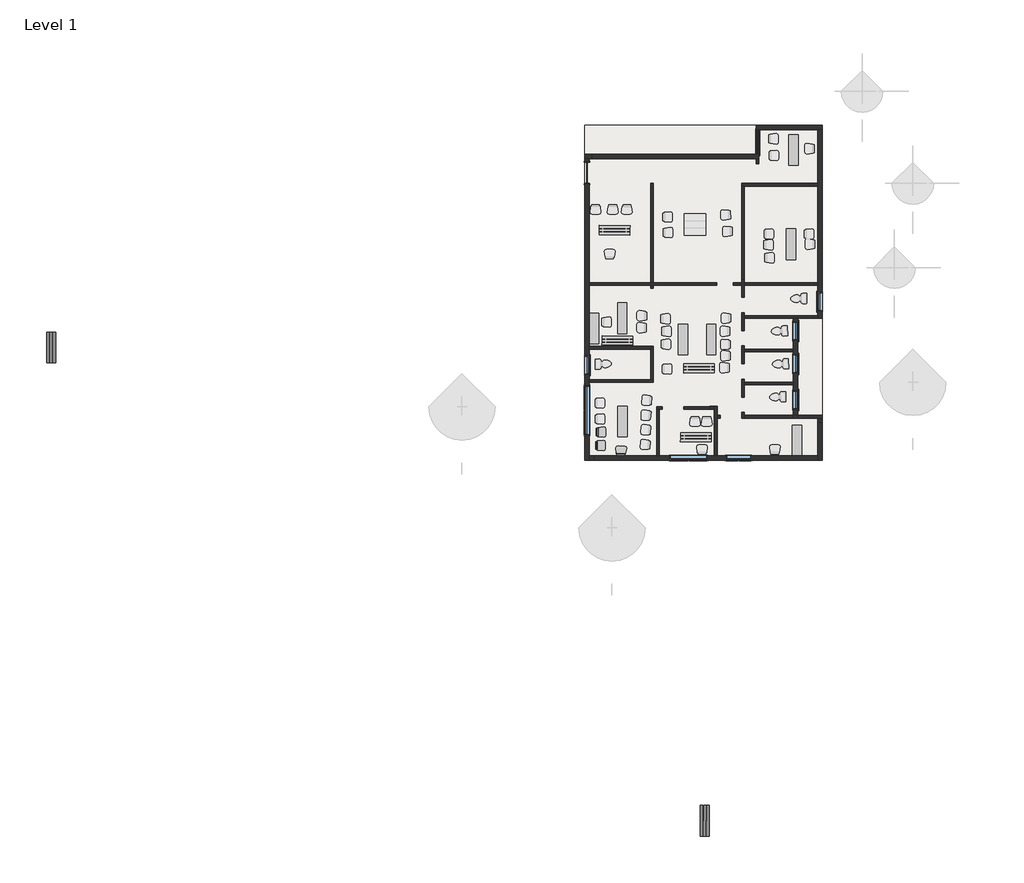
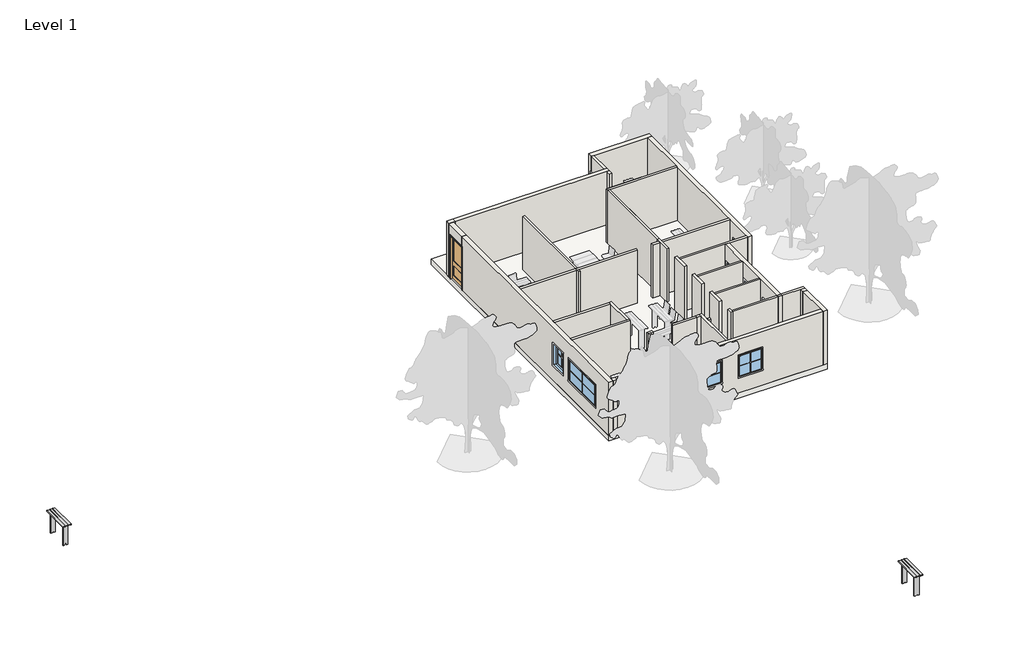
# One storey, part 1 of 2: 46 walls, 9 windows, 5 furniture elements, 1 door, 1 slab.
"""IFC4 building model written with IfcOpenShell, lengths in millimetres."""

from ifc_helpers import new_model, si_unit, frame, origin, origin_with_axes, place, context, project, spatial, polyline, outline, extrude, faceted_brep, transform, mapped, element, save
from components import door_07f5c701, furniture_f7008d8d, chair_desk_chair_desk_7ad88740, window_fixed_2_d4a0c5b4, window_fixed_3_f41792bd, window_fixed_5_cc3256ea, window_fixed_8_9704bb16, window_fixed_9_035f8342

model = new_model("IFC4")

# Units and contexts
model_context = context("Model", 3, world=origin())
ifc_project = project(units=[si_unit("LENGTHUNIT", "METRE", prefix="MILLI")], contexts=[model_context])

# Site, building, storey
site = spatial("IfcSite", under=ifc_project)
building = spatial("IfcBuilding", under=site)
storey = spatial("IfcBuildingStorey", under=building, Name="Level 1", Elevation=0.0)

# Door
placement = place(None, origin())
door_shape = door_07f5c701(model_context)
element("IfcDoor", 1, ObjectType="Door-Interior-Single-Pocket-2_Panel-Wood : 42\" x 96\"", at=placement, inside=storey, context=model_context, shape_type="MappedRepresentation", body=[
    mapped(door_shape, transform((1384.3, 26568.4, 0.0), x_axis=(0.0, -1.0, 0.0), y_axis=(1.0, 0.0, 0.0), z_axis=(0.0, 0.0, 1.0))),
])

# Furniture
furniture_shape = furniture_f7008d8d(model_context)
element("IfcFurniture", 2, ObjectType="Bench-Locker Room : 48\" x 18\" x 14\"", at=placement, inside=storey, context=model_context, shape_type="MappedRepresentation", body=[
    mapped(furniture_shape, transform((-25423.3983688, 18061.4041391, 0.0), x_axis=(0.0, 1.0, 0.0), y_axis=(-1.0, 0.0, 0.0), z_axis=(0.0, 0.0, 1.0))),
])
element("IfcFurniture", 3, ObjectType="Bench-Locker Room : 48\" x 18\" x 14\"", at=placement, inside=storey, context=model_context, shape_type="MappedRepresentation", body=[
    mapped(furniture_shape, transform((7417.2524983, -5769.7183685, 0.0), x_axis=(-0.004811439454211425, -0.9999884249581985, 0.0), y_axis=(0.9999884249581985, -0.004811439454211425, 0.0), z_axis=(0.0, 0.0, 1.0))),
])
chair_desk_chair_desk_shape = chair_desk_chair_desk_7ad88740(model_context)
element("IfcFurniture", 4, ObjectType="Chair-Desk : Chair-Desk", at=placement, inside=storey, context=model_context, shape_type="MappedRepresentation", body=[
    mapped(chair_desk_chair_desk_shape, transform((1917.2646776, 13701.8247599, 0.0), x_axis=(0.0, -1.0, 0.0), y_axis=(1.0, 0.0, 0.0), z_axis=(0.0, 0.0, 1.0))),
])
element("IfcFurniture", 5, ObjectType="Chair-Desk : Chair-Desk", at=placement, inside=storey, context=model_context, shape_type="MappedRepresentation", body=[
    mapped(chair_desk_chair_desk_shape, transform((1889.1210098, 13035.1530931, 0.0), x_axis=(0.0, -1.0, 0.0), y_axis=(1.0, 0.0, 0.0), z_axis=(0.0, 0.0, 1.0))),
])
element("IfcFurniture", 6, ObjectType="Chair-Desk : Chair-Desk", at=placement, inside=storey, context=model_context, shape_type="MappedRepresentation", body=[
    mapped(chair_desk_chair_desk_shape, transform((3069.589979, 12617.2374558, 0.0), x_axis=(0.9977976465817522, -0.066331413944804, 0.0), y_axis=(0.066331413944804, 0.9977976465817522, 0.0), z_axis=(0.0, 0.0, 1.0))),
])

# Slab
element("IfcSlab", 7, ObjectType="Generic - 12\"", at=placement, inside=storey, context=model_context, shape_type="SweptSolid", body=[
    extrude(outline(polyline([(1270.0, 28956.0), (13081.0, 28956.0), (13081.0, 12293.6), (1270.0, 12293.6), (1270.0, 28956.0)])), frame((0.0, 0.0, -304.8), z_axis=(0.0, 0.0, 1.0), x_axis=(1.0, 0.0, 0.0)), (0.0, 0.0, 1.0), 304.8),
])

# Walls
element("IfcWall", 8, at=placement, inside=storey, context=model_context, shape_type="Brep", body=[
    faceted_brep([(7493.0, 14985.1789567, 0.0), (7493.0, 14960.6, 0.0), (7493.0, 14833.6, 0.0), (7493.0, 14833.6, 3048.0), (7493.0, 14960.6, 3048.0), (7493.0, 14985.1789567, 3048.0), (7721.6, 14985.1789567, 0.0), (7721.6, 14985.1789567, 3048.0), (7721.6, 14833.6, 3048.0), (7721.6, 14833.6, 0.0)], [[[0, 1, 2, 3, 4, 5]], [[6, 7, 8, 9]], [[2, 1, 0, 6, 9]], [[0, 5, 7, 6]], [[3, 2, 9, 8]], [[5, 4, 3, 8, 7]]]),
])
element("IfcWall", 9, at=placement, inside=storey, context=model_context, shape_type="SweptSolid", body=[
    extrude(outline(polyline([(7493.0, 14960.6), (7493.0, 14985.1789567), (7721.6, 14985.1789567), (7721.6, 14960.6), (7493.0, 14960.6)])), origin_with_axes(), (0.0, 0.0, 1.0), 3048.0),
])
element("IfcWall", 10, ObjectType="5\"", at=placement, inside=storey, context=model_context, shape_type="Brep", body=[
    faceted_brep([(12852.4, 19481.8, 0.0), (9194.8, 19481.8, 0.0), (9194.8, 19481.8, 3048.0), (12852.4, 19481.8, 3048.0), (12852.4, 19354.8, 0.0), (12852.4, 19354.8, 3048.0), (11861.8, 19354.8, 3048.0), (11633.2, 19354.8, 3048.0), (9194.8, 19354.8, 3048.0), (9194.8, 19354.8, 0.0), (11633.2, 19354.8, 0.0), (11861.8, 19354.8, 0.0)], [[[0, 1, 2, 3]], [[4, 5, 6, 7, 8, 9, 10, 11]], [[1, 0, 4, 11, 10, 9]], [[0, 3, 5, 4]], [[2, 1, 9, 8]], [[3, 2, 8, 7, 6, 5]]]),
])
element("IfcWall", 11, ObjectType="5\"", at=placement, inside=storey, context=model_context, shape_type="Brep", body=[
    faceted_brep([(9067.8, 19634.2, 0.0), (9067.8, 18745.2, 0.0), (9067.8, 18745.2, 3048.0), (9067.8, 19634.2, 3048.0), (9194.8, 19634.2, 0.0), (9194.8, 19634.2, 3048.0), (9194.8, 19481.8, 3048.0), (9194.8, 19354.8, 3048.0), (9194.8, 18745.2, 3048.0), (9194.8, 18745.2, 0.0), (9194.8, 19354.8, 0.0), (9194.8, 19481.8, 0.0)], [[[0, 1, 2, 3]], [[4, 5, 6, 7, 8, 9, 10, 11]], [[1, 0, 4, 11, 10, 9]], [[2, 1, 9, 8]], [[0, 3, 5, 4]], [[3, 2, 8, 7, 6, 5]]]),
])
element("IfcWall", 12, ObjectType="5\"", at=placement, inside=storey, context=model_context, shape_type="SweptSolid", body=[
    extrude(outline(polyline([(9067.8, 20396.2), (9067.8, 21285.2), (9194.8, 21285.2), (9194.8, 20396.2), (9067.8, 20396.2)])), origin_with_axes(), (0.0, 0.0, 1.0), 3048.0),
])
element("IfcWall", 13, ObjectType="5\"", at=placement, inside=storey, context=model_context, shape_type="Brep", body=[
    faceted_brep([(12852.4, 26060.4, 0.0), (9067.8, 26060.4, 0.0), (9067.8, 26060.4, 3048.0), (12852.4, 26060.4, 3048.0), (12852.4, 25933.4, 0.0), (12852.4, 25933.4, 3048.0), (9194.8, 25933.4, 3048.0), (9067.8, 25933.4, 3048.0), (9067.8, 25933.4, 0.0), (9194.8, 25933.4, 0.0)], [[[0, 1, 2, 3]], [[4, 5, 6, 7, 8, 9]], [[1, 0, 4, 9, 8]], [[0, 3, 5, 4]], [[2, 1, 8, 7]], [[3, 2, 7, 6, 5]]]),
])
element("IfcWall", 14, ObjectType="5\"", at=placement, inside=storey, context=model_context, shape_type="SweptSolid", body=[
    extrude(outline(polyline([(9067.8, 22352.0), (9067.8, 25933.4), (9194.8, 25933.4), (9194.8, 22352.0), (9067.8, 22352.0)])), origin_with_axes(), (0.0, 0.0, 1.0), 3048.0),
])
element("IfcWall", 15, ObjectType="5\"", at=placement, inside=storey, context=model_context, shape_type="SweptSolid", body=[
    extrude(outline(polyline([(9194.8, 17830.8), (11633.2, 17830.8), (11633.2, 17703.8), (9194.8, 17703.8), (9194.8, 17830.8)])), origin_with_axes(), (0.0, 0.0, 1.0), 3048.0),
])
element("IfcWall", 16, ObjectType="5\"", at=placement, inside=storey, context=model_context, shape_type="Brep", body=[
    faceted_brep([(9067.8, 17983.2, 0.0), (9067.8, 17094.2, 0.0), (9067.8, 17094.2, 3048.0), (9067.8, 17983.2, 3048.0), (9194.8, 17983.2, 0.0), (9194.8, 17983.2, 3048.0), (9194.8, 17830.8, 3048.0), (9194.8, 17703.8, 3048.0), (9194.8, 17094.2, 3048.0), (9194.8, 17094.2, 0.0), (9194.8, 17703.8, 0.0), (9194.8, 17830.8, 0.0)], [[[0, 1, 2, 3]], [[4, 5, 6, 7, 8, 9, 10, 11]], [[1, 0, 4, 11, 10, 9]], [[2, 1, 9, 8]], [[0, 3, 5, 4]], [[3, 2, 8, 7, 6, 5]]]),
])
element("IfcWall", 17, ObjectType="5\"", at=placement, inside=storey, context=model_context, shape_type="SweptSolid", body=[
    extrude(outline(polyline([(9194.8, 16179.8), (11633.2, 16179.8), (11633.2, 16052.8), (9194.8, 16052.8), (9194.8, 16179.8)])), origin_with_axes(), (0.0, 0.0, 1.0), 3048.0),
])
element("IfcWall", 18, ObjectType="5\"", at=placement, inside=storey, context=model_context, shape_type="Brep", body=[
    faceted_brep([(9067.8, 16332.2, 0.0), (9067.8, 15443.2, 0.0), (9067.8, 15443.2, 3048.0), (9067.8, 16332.2, 3048.0), (9194.8, 16332.2, 0.0), (9194.8, 16332.2, 3048.0), (9194.8, 16179.8, 3048.0), (9194.8, 16052.8, 3048.0), (9194.8, 15443.2, 3048.0), (9194.8, 15443.2, 0.0), (9194.8, 16052.8, 0.0), (9194.8, 16179.8, 0.0)], [[[0, 1, 2, 3]], [[4, 5, 6, 7, 8, 9, 10, 11]], [[1, 0, 4, 11, 10, 9]], [[2, 1, 9, 8]], [[0, 3, 5, 4]], [[3, 2, 8, 7, 6, 5]]]),
])
element("IfcWall", 19, ObjectType="5\"", at=placement, inside=storey, context=model_context, shape_type="Brep", body=[
    faceted_brep([(13081.0, 14528.8, 0.0), (11861.8, 14528.8, 0.0), (11633.2, 14528.8, 0.0), (9194.8, 14528.8, 0.0), (9194.8, 14528.8, 3048.0), (11633.2, 14528.8, 3048.0), (11861.8, 14528.8, 3048.0), (13081.0, 14528.8, 3048.0), (13081.0, 14401.8, 0.0), (13081.0, 14401.8, 3048.0), (9194.8, 14401.8, 3048.0), (9194.8, 14401.8, 0.0)], [[[0, 1, 2, 3, 4, 5, 6, 7]], [[8, 9, 10, 11]], [[3, 2, 1, 0, 8, 11]], [[0, 7, 9, 8]], [[4, 3, 11, 10]], [[7, 6, 5, 4, 10, 9]]]),
])
element("IfcWall", 20, ObjectType="5\"", at=placement, inside=storey, context=model_context, shape_type="Brep", body=[
    faceted_brep([(9067.8, 14681.2, 0.0), (9067.8, 14401.8, 0.0), (9067.8, 14401.8, 3048.0), (9067.8, 14681.2, 3048.0), (9194.8, 14681.2, 0.0), (9194.8, 14681.2, 3048.0), (9194.8, 14528.8, 3048.0), (9194.8, 14401.8, 3048.0), (9194.8, 14401.8, 0.0), (9194.8, 14528.8, 0.0)], [[[0, 1, 2, 3]], [[4, 5, 6, 7, 8, 9]], [[1, 0, 4, 9, 8]], [[0, 3, 5, 4]], [[2, 1, 8, 7]], [[3, 2, 7, 6, 5]]]),
])
element("IfcWall", 21, ObjectType="5\"", at=placement, inside=storey, context=model_context, shape_type="SweptSolid", body=[
    extrude(outline(polyline([(1498.6, 21132.8), (7844.2592865, 21132.8), (7844.2592865, 21005.8), (1498.6, 21005.8), (1498.6, 21132.8)])), origin_with_axes(), (0.0, 0.0, 1.0), 3048.0),
])
element("IfcWall", 22, ObjectType="5\"", at=placement, inside=storey, context=model_context, shape_type="SweptSolid", body=[
    extrude(outline(polyline([(4546.6, 20853.4004015), (4546.6, 26060.4), (4673.6, 26060.4), (4673.6, 20853.4004015), (4546.6, 20853.4004015)])), origin_with_axes(), (0.0, 0.0, 1.0), 3048.0),
])
element("IfcWall", 23, ObjectType="5\"", at=placement, inside=storey, context=model_context, shape_type="Brep", body=[
    faceted_brep([(5130.8, 14960.6, 0.0), (4851.4, 14960.6, 0.0), (4851.4, 14960.6, 3048.0), (5130.8, 14960.6, 3048.0), (5130.8, 14833.6, 0.0), (5130.8, 14833.6, 3048.0), (4978.4, 14833.6, 3048.0), (4851.4, 14833.6, 3048.0), (4851.4, 14833.6, 0.0), (4978.4, 14833.6, 0.0)], [[[0, 1, 2, 3]], [[4, 5, 6, 7, 8, 9]], [[1, 0, 4, 9, 8]], [[0, 3, 5, 4]], [[2, 1, 8, 7]], [[3, 2, 7, 6, 5]]]),
])
element("IfcWall", 24, ObjectType="5\"", at=placement, inside=storey, context=model_context, shape_type="SweptSolid", body=[
    extrude(outline(polyline([(4851.4, 12522.2), (4851.4, 14833.6), (4978.4, 14833.6), (4978.4, 12522.2), (4851.4, 12522.2)])), origin_with_axes(), (0.0, 0.0, 1.0), 3048.0),
])
element("IfcWall", 25, ObjectType="5\"", at=placement, inside=storey, context=model_context, shape_type="Brep", body=[
    faceted_brep([(7848.6, 12522.2, 0.0), (7848.6, 14401.8, 0.0), (7848.6, 14528.8, 0.0), (7848.6, 14985.1789567, 0.0), (7848.6, 14985.1789567, 3048.0), (7848.6, 14528.8, 3048.0), (7848.6, 14401.8, 3048.0), (7848.6, 12522.2, 3048.0), (7721.6, 12522.2, 0.0), (7721.6, 12522.2, 3048.0), (7721.6, 14985.1789567, 3048.0), (7721.6, 14985.1789567, 0.0)], [[[0, 1, 2, 3, 4, 5, 6, 7]], [[8, 9, 10, 11]], [[3, 2, 1, 0, 8, 11]], [[4, 3, 11, 10]], [[0, 7, 9, 8]], [[7, 6, 5, 4, 10, 9]]]),
])
element("IfcWall", 26, ObjectType="5\"", at=placement, inside=storey, context=model_context, shape_type="SweptSolid", body=[
    extrude(outline(polyline([(6197.6, 14960.6), (7493.0, 14960.6), (7493.0, 14833.6), (6197.6, 14833.6), (6197.6, 14960.6)])), origin_with_axes(), (0.0, 0.0, 1.0), 3048.0),
])
element("IfcWall", 27, ObjectType="5\"", at=placement, inside=storey, context=model_context, shape_type="SweptSolid", body=[
    extrude(outline(polyline([(9804.4, 27508.2), (9804.4, 28727.4), (9931.4, 28727.4), (9931.4, 27508.2), (9804.4, 27508.2)])), origin_with_axes(), (0.0, 0.0, 1.0), 914.4),
    extrude(outline(polyline([(9804.4, 27508.2), (9804.4, 28727.4), (9931.4, 28727.4), (9931.4, 27508.2), (9804.4, 27508.2)])), frame((0.0, 0.0, 2133.6), z_axis=(0.0, 0.0, 1.0), x_axis=(1.0, 0.0, 0.0)), (0.0, 0.0, 1.0), 914.4),
])
element("IfcWall", 28, ObjectType="5\"", at=placement, inside=storey, context=model_context, shape_type="SweptSolid", body=[
    extrude(outline(polyline([(7874.0, 14401.8), (7874.0, 14528.8), (8001.0, 14528.8), (8001.0, 14401.8), (7874.0, 14401.8)])), origin_with_axes(), (0.0, 0.0, 1.0), 3048.0),
])
element("IfcWall", 29, ObjectType="5\"", at=placement, inside=storey, context=model_context, shape_type="SweptSolid", body=[
    extrude(outline(polyline([(7848.6, 14528.8), (7874.0, 14528.8), (7874.0, 14401.8), (7848.6, 14401.8), (7848.6, 14528.8)])), origin_with_axes(), (0.0, 0.0, 1.0), 3048.0),
])
element("IfcWall", 30, ObjectType="9\"", at=placement, inside=storey, context=model_context, shape_type="SweptSolid", body=[
    extrude(outline(polyline([(27279.6, 3048.0), (27279.6, 0.0), (27127.2, 0.0), (27127.2, 2463.8), (26060.4, 2463.8), (26060.4, 3048.0), (27279.6, 3048.0)])), frame((1270.0, 0.0, 0.0), z_axis=(1.0, 0.0, 0.0), x_axis=(0.0, 1.0, 0.0)), (0.0, 0.0, 1.0), 228.6),
])
element("IfcWall", 31, ObjectType="9\"", at=placement, inside=storey, context=model_context, shape_type="Brep", body=[
    faceted_brep([(1270.0, 12293.6, 0.0), (1270.0, 12293.6, 3048.0), (1270.0, 26060.4, 3048.0), (1270.0, 26060.4, 2463.8), (1270.0, 26035.0, 2463.8), (1270.0, 26035.0, 0.0), (1270.0, 16572.1631818, 2133.6), (1270.0, 16572.1631818, 914.4), (1270.0, 17486.5631818, 914.4), (1270.0, 17486.5631818, 2133.6), (1270.0, 16002.6980131, 2133.6), (1270.0, 13564.2980131, 2133.6), (1270.0, 13564.2980131, 914.4), (1270.0, 16002.6980131, 914.4), (1498.6, 12293.6, 3048.0), (1498.6, 12293.6, 0.0), (1498.6, 16179.8, 0.0), (1498.6, 16306.8, 0.0), (1498.6, 17830.8, 0.0), (1498.6, 17957.8, 0.0), (1498.6, 21005.8, 0.0), (1498.6, 21132.8, 0.0), (1498.6, 26035.0, 0.0), (1498.6, 26035.0, 2463.8), (1498.6, 26060.4, 2463.8), (1498.6, 26060.4, 3048.0), (1498.6, 21132.8, 3048.0), (1498.6, 21005.8, 3048.0), (1498.6, 17957.8, 3048.0), (1498.6, 17830.8, 3048.0), (1498.6, 16306.8, 3048.0), (1498.6, 16179.8, 3048.0), (1498.6, 16572.1631818, 2133.6), (1498.6, 17486.5631818, 2133.6), (1498.6, 17486.5631818, 914.4), (1498.6, 16572.1631818, 914.4), (1498.6, 16002.6980131, 2133.6), (1498.6, 16002.6980131, 914.4), (1498.6, 13564.2980131, 914.4), (1498.6, 13564.2980131, 2133.6), (1363.6625, 26035.0, 0.0), (1363.6625, 24968.2, 0.0), (1404.9375, 24968.2, 0.0), (1404.9375, 26035.0, 0.0), (1404.9375, 24968.2, 2463.8), (1363.6625, 24968.2, 2463.8), (1363.6625, 26035.0, 2463.8), (1404.9375, 26035.0, 2463.8)], [[[0, 1, 2, 3, 4, 5], [6, 7, 8, 9], [10, 11, 12, 13]], [[14, 15, 16, 17, 18, 19, 20, 21, 22, 23, 24, 25, 26, 27, 28, 29, 30, 31], [32, 33, 34, 35], [36, 37, 38, 39]], [[15, 0, 5, 40, 41, 42, 43, 22, 21, 20, 19, 18, 17, 16]], [[1, 0, 15, 14]], [[2, 25, 24, 3]], [[7, 6, 32, 35]], [[8, 7, 35, 34]], [[9, 8, 34, 33]], [[6, 9, 33, 32]], [[37, 36, 10, 13]], [[38, 37, 13, 12]], [[39, 38, 12, 11]], [[36, 39, 11, 10]], [[44, 45, 46, 4, 3, 24, 23, 47]], [[44, 47, 43, 42]], [[47, 23, 22, 43]], [[4, 46, 40, 5]], [[46, 45, 41, 40]], [[45, 44, 42, 41]], [[25, 2, 1, 14, 31, 30, 29, 28, 27, 26]]]),
])
element("IfcWall", 32, ObjectType="9\"", at=placement, inside=storey, context=model_context, shape_type="SweptSolid", body=[
    extrude(outline(polyline([(1727.1306168, 12522.2), (1727.1306168, 12293.6), (1498.5306168, 12293.6), (1498.5306168, 12522.2), (1727.1306168, 12522.2)])), origin_with_axes(), (0.0, 0.0, 1.0), 3048.0),
])
element("IfcWall", 33, ObjectType="9\"", at=placement, inside=storey, context=model_context, shape_type="Brep", body=[
    faceted_brep([(9804.4, 28727.4, 0.0), (9931.4, 28727.4, 0.0), (12852.4, 28727.4, 0.0), (13081.0, 28727.4, 0.0), (13081.0, 28727.4, 3048.0), (12852.4, 28727.4, 3048.0), (9931.4, 28727.4, 3048.0), (9804.4, 28727.4, 3048.0), (9804.4, 28727.4, 2133.6), (9804.4, 28727.4, 914.4), (9804.4, 28956.0, 0.0), (9804.4, 28956.0, 3048.0), (13081.0, 28956.0, 3048.0), (13081.0, 28956.0, 0.0)], [[[0, 1, 2, 3, 4, 5, 6, 7, 8, 9]], [[10, 11, 12, 13]], [[3, 2, 1, 0, 10, 13]], [[4, 3, 13, 12]], [[0, 9, 8, 7, 11, 10]], [[7, 6, 5, 4, 12, 11]]]),
])
element("IfcWall", 34, ObjectType="9\"", at=placement, inside=storey, context=model_context, shape_type="Brep", body=[
    faceted_brep([(12852.4, 28727.4, 0.0), (12852.4, 26060.4, 0.0), (12852.4, 25933.4, 0.0), (12852.4, 21132.8, 0.0), (12852.4, 21005.8, 0.0), (12852.4, 19481.8, 0.0), (12852.4, 19354.8, 0.0), (12852.4, 19354.8, 3048.0), (12852.4, 19481.8, 3048.0), (12852.4, 21005.8, 3048.0), (12852.4, 21132.8, 3048.0), (12852.4, 25933.4, 3048.0), (12852.4, 26060.4, 3048.0), (12852.4, 28727.4, 3048.0), (12852.4, 20643.2468811, 2133.6), (12852.4, 19728.8468811, 2133.6), (12852.4, 19728.8468811, 914.4), (12852.4, 20643.2468811, 914.4), (13081.0, 28727.4, 0.0), (13081.0, 28727.4, 3048.0), (13081.0, 19354.8, 3048.0), (13081.0, 19354.8, 0.0), (13081.0, 20643.2468811, 2133.6), (13081.0, 20643.2468811, 914.4), (13081.0, 19728.8468811, 914.4), (13081.0, 19728.8468811, 2133.6)], [[[0, 1, 2, 3, 4, 5, 6, 7, 8, 9, 10, 11, 12, 13], [14, 15, 16, 17]], [[18, 19, 20, 21], [22, 23, 24, 25]], [[6, 5, 4, 3, 2, 1, 0, 18, 21]], [[0, 13, 19, 18]], [[7, 6, 21, 20]], [[23, 22, 14, 17]], [[24, 23, 17, 16]], [[25, 24, 16, 15]], [[22, 25, 15, 14]], [[13, 12, 11, 10, 9, 8, 7, 20, 19]]]),
])
element("IfcWall", 35, ObjectType="9\"", at=placement, inside=storey, context=model_context, shape_type="Brep", body=[
    faceted_brep([(11633.2, 19354.8, 0.0), (11633.2, 17830.8, 0.0), (11633.2, 17703.8, 0.0), (11633.2, 16179.8, 0.0), (11633.2, 16052.8, 0.0), (11633.2, 14528.8, 0.0), (11633.2, 14528.8, 3048.0), (11633.2, 16052.8, 3048.0), (11633.2, 16179.8, 3048.0), (11633.2, 17703.8, 3048.0), (11633.2, 17830.8, 3048.0), (11633.2, 19354.8, 3048.0), (11633.2, 18268.95, 2133.6), (11633.2, 18268.95, 914.4), (11633.2, 19183.35, 914.4), (11633.2, 19183.35, 2133.6), (11633.2, 14842.6267416, 2133.6), (11633.2, 14842.6267416, 914.4), (11633.2, 15757.0267416, 914.4), (11633.2, 15757.0267416, 2133.6), (11633.2, 16635.1067598, 2133.6), (11633.2, 16635.1067598, 914.4), (11633.2, 17549.5067598, 914.4), (11633.2, 17549.5067598, 2133.6), (11861.8, 19354.8, 0.0), (11861.8, 19354.8, 3048.0), (11861.8, 14528.8, 3048.0), (11861.8, 14528.8, 0.0), (11861.8, 18268.95, 2133.6), (11861.8, 19183.35, 2133.6), (11861.8, 19183.35, 914.4), (11861.8, 18268.95, 914.4), (11861.8, 14842.6267416, 2133.6), (11861.8, 15757.0267416, 2133.6), (11861.8, 15757.0267416, 914.4), (11861.8, 14842.6267416, 914.4), (11861.8, 16635.1067598, 2133.6), (11861.8, 17549.5067598, 2133.6), (11861.8, 17549.5067598, 914.4), (11861.8, 16635.1067598, 914.4)], [[[0, 1, 2, 3, 4, 5, 6, 7, 8, 9, 10, 11], [12, 13, 14, 15], [16, 17, 18, 19], [20, 21, 22, 23]], [[24, 25, 26, 27], [28, 29, 30, 31], [32, 33, 34, 35], [36, 37, 38, 39]], [[5, 4, 3, 2, 1, 0, 24, 27]], [[0, 11, 25, 24]], [[6, 5, 27, 26]], [[13, 12, 28, 31]], [[14, 13, 31, 30]], [[15, 14, 30, 29]], [[12, 15, 29, 28]], [[17, 16, 32, 35]], [[18, 17, 35, 34]], [[19, 18, 34, 33]], [[16, 19, 33, 32]], [[21, 20, 36, 39]], [[22, 21, 39, 38]], [[23, 22, 38, 37]], [[20, 23, 37, 36]], [[11, 10, 9, 8, 7, 6, 26, 25]]]),
])
element("IfcWall", 36, ObjectType="9\"", at=placement, inside=storey, context=model_context, shape_type="SweptSolid", body=[
    extrude(outline(polyline([(11633.2, 14401.8), (11633.2, 14528.8), (11861.8, 14528.8), (11861.8, 14401.8), (11633.2, 14401.8)])), origin_with_axes(), (0.0, 0.0, 1.0), 3048.0),
])
element("IfcWall", 37, ObjectType="9\"", at=placement, inside=storey, context=model_context, shape_type="SweptSolid", body=[
    extrude(outline(polyline([(13081.0, 14173.2), (12852.4, 14173.2), (12852.4, 14401.8), (13081.0, 14401.8), (13081.0, 14173.2)])), origin_with_axes(), (0.0, 0.0, 1.0), 3048.0),
])
element("IfcWall", 38, ObjectType="9\"", at=placement, inside=storey, context=model_context, shape_type="Brep", body=[
    faceted_brep([(12852.4, 14173.2, 0.0), (12852.4, 12522.2, 0.0), (12852.4, 12293.6, 0.0), (12852.4, 12293.6, 3048.0), (12852.4, 12522.2, 3048.0), (12852.4, 14173.2, 3048.0), (13081.0, 14173.2, 0.0), (13081.0, 14173.2, 3048.0), (13081.0, 12293.6, 3048.0), (13081.0, 12293.6, 0.0)], [[[0, 1, 2, 3, 4, 5]], [[6, 7, 8, 9]], [[2, 1, 0, 6, 9]], [[0, 5, 7, 6]], [[3, 2, 9, 8]], [[5, 4, 3, 8, 7]]]),
])
element("IfcWall", 39, ObjectType="9\"", at=placement, inside=storey, context=model_context, shape_type="Brep", body=[
    faceted_brep([(12852.4, 12522.2, 0.0), (7848.6, 12522.2, 0.0), (7721.6, 12522.2, 0.0), (4978.4, 12522.2, 0.0), (4851.4, 12522.2, 0.0), (1727.1306168, 12522.2, 0.0), (1727.1306168, 12522.2, 3048.0), (4851.4, 12522.2, 3048.0), (4978.4, 12522.2, 3048.0), (7721.6, 12522.2, 3048.0), (7848.6, 12522.2, 3048.0), (12852.4, 12522.2, 3048.0), (5511.8, 12522.2, 2133.6), (5511.8, 12522.2, 914.4), (7340.6, 12522.2, 914.4), (7340.6, 12522.2, 2133.6), (8312.15, 12522.2, 2133.6), (8312.15, 12522.2, 914.4), (9531.35, 12522.2, 914.4), (9531.35, 12522.2, 2133.6), (1727.1306168, 12293.6, 0.0), (12852.4, 12293.6, 0.0), (12852.4, 12293.6, 3048.0), (1727.1306168, 12293.6, 3048.0), (5511.8, 12293.6, 914.4), (5511.8, 12293.6, 2133.6), (7340.6, 12293.6, 2133.6), (7340.6, 12293.6, 914.4), (8312.15, 12293.6, 914.4), (8312.15, 12293.6, 2133.6), (9531.35, 12293.6, 2133.6), (9531.35, 12293.6, 914.4)], [[[0, 1, 2, 3, 4, 5, 6, 7, 8, 9, 10, 11], [12, 13, 14, 15], [16, 17, 18, 19]], [[20, 21, 22, 23], [24, 25, 26, 27], [28, 29, 30, 31]], [[5, 4, 3, 2, 1, 0, 21, 20]], [[0, 11, 22, 21]], [[6, 5, 20, 23]], [[24, 13, 12, 25]], [[13, 24, 27, 14]], [[14, 27, 26, 15]], [[15, 26, 25, 12]], [[16, 29, 28, 17]], [[17, 28, 31, 18]], [[18, 31, 30, 19]], [[29, 16, 19, 30]], [[11, 10, 9, 8, 7, 6, 23, 22]]]),
])
element("IfcWall", 40, ObjectType="9\"", at=placement, inside=storey, context=model_context, shape_type="Brep", body=[
    faceted_brep([(1612.9, 27279.6, 0.0), (9931.4, 27279.6, 0.0), (9931.4, 27279.6, 3048.0), (1612.9, 27279.6, 3048.0), (1612.9, 27508.2, 0.0), (1612.9, 27508.2, 3048.0), (9804.4, 27508.2, 3048.0), (9931.4, 27508.2, 3048.0), (9931.4, 27508.2, 2133.6), (9931.4, 27508.2, 914.4), (9931.4, 27508.2, 0.0), (9804.4, 27508.2, 0.0)], [[[0, 1, 2, 3]], [[4, 5, 6, 7, 8, 9, 10, 11]], [[1, 0, 4, 11, 10]], [[0, 3, 5, 4]], [[2, 1, 10, 9, 8, 7]], [[3, 2, 7, 6, 5]]]),
])
element("IfcWall", 41, ObjectType="9\"", at=placement, inside=storey, context=model_context, shape_type="Brep", body=[
    faceted_brep([(1612.9, 27508.2, 0.0), (1270.0, 27508.2, 0.0), (1270.0, 27508.2, 3048.0), (1612.9, 27508.2, 3048.0), (1612.9, 27279.6, 0.0), (1612.9, 27279.6, 3048.0), (1498.6, 27279.6, 3048.0), (1270.0, 27279.6, 3048.0), (1270.0, 27279.6, 0.0), (1498.6, 27279.6, 0.0)], [[[0, 1, 2, 3]], [[4, 5, 6, 7, 8, 9]], [[1, 0, 4, 9, 8]], [[0, 3, 5, 4]], [[2, 1, 8, 7]], [[3, 2, 7, 6, 5]]]),
])
element("IfcWall", 42, ObjectType="9\"", at=placement, inside=storey, context=model_context, shape_type="SweptSolid", body=[
    extrude(outline(polyline([(9931.4, 27051.0), (9804.4, 27051.0), (9804.4, 27279.6), (9931.4, 27279.6), (9931.4, 27051.0)])), origin_with_axes(), (0.0, 0.0, 1.0), 3048.0),
])
element("IfcWall", 43, ObjectType="double5\"", at=placement, inside=storey, context=model_context, shape_type="Brep", body=[
    faceted_brep([(12852.4, 19481.8, 0.0), (9194.8, 19481.8, 0.0), (9194.8, 19481.8, 3048.0), (12852.4, 19481.8, 3048.0), (12852.4, 19354.8, 0.0), (12852.4, 19354.8, 3048.0), (11861.8, 19354.8, 3048.0), (11633.2, 19354.8, 3048.0), (9194.8, 19354.8, 3048.0), (9194.8, 19354.8, 0.0), (11633.2, 19354.8, 0.0), (11861.8, 19354.8, 0.0)], [[[0, 1, 2, 3]], [[4, 5, 6, 7, 8, 9, 10, 11]], [[1, 0, 4, 11, 10, 9]], [[0, 3, 5, 4]], [[2, 1, 9, 8]], [[3, 2, 8, 7, 6, 5]]]),
])
element("IfcWall", 44, ObjectType="double5\"", at=placement, inside=storey, context=model_context, shape_type="Brep", body=[
    faceted_brep([(12852.4, 19481.8, 0.0), (9194.8, 19481.8, 0.0), (9194.8, 19481.8, 3048.0), (12852.4, 19481.8, 3048.0), (12852.4, 19354.8, 0.0), (12852.4, 19354.8, 3048.0), (11861.8, 19354.8, 3048.0), (11633.2, 19354.8, 3048.0), (9194.8, 19354.8, 3048.0), (9194.8, 19354.8, 0.0), (11633.2, 19354.8, 0.0), (11861.8, 19354.8, 0.0)], [[[0, 1, 2, 3]], [[4, 5, 6, 7, 8, 9, 10, 11]], [[1, 0, 4, 11, 10, 9]], [[0, 3, 5, 4]], [[2, 1, 9, 8]], [[3, 2, 8, 7, 6, 5]]]),
])
element("IfcWall", 45, ObjectType="double5\"", at=placement, inside=storey, context=model_context, shape_type="Brep", body=[
    faceted_brep([(9067.8, 19634.2, 0.0), (9067.8, 18745.0941593, 0.0), (9067.8, 18745.0941593, 3048.0), (9067.8, 19634.2, 3048.0), (9194.8, 19634.2, 0.0), (9194.8, 19634.2, 3048.0), (9194.8, 19481.8, 3048.0), (9194.8, 19354.8, 3048.0), (9194.8, 18745.0941593, 3048.0), (9194.8, 18745.0941593, 0.0), (9194.8, 19354.8, 0.0), (9194.8, 19481.8, 0.0)], [[[0, 1, 2, 3]], [[4, 5, 6, 7, 8, 9, 10, 11]], [[1, 0, 4, 11, 10, 9]], [[2, 1, 9, 8]], [[0, 3, 5, 4]], [[3, 2, 8, 7, 6, 5]]]),
])
element("IfcWall", 46, ObjectType="double5\"", at=placement, inside=storey, context=model_context, shape_type="Brep", body=[
    faceted_brep([(12852.4, 19481.8, 0.0), (9194.8, 19481.8, 0.0), (9194.8, 19481.8, 3048.0), (12852.4, 19481.8, 3048.0), (12852.4, 19354.8, 0.0), (12852.4, 19354.8, 3048.0), (11861.8, 19354.8, 3048.0), (11633.2, 19354.8, 3048.0), (9194.8, 19354.8, 3048.0), (9194.8, 19354.8, 0.0), (11633.2, 19354.8, 0.0), (11861.8, 19354.8, 0.0)], [[[0, 1, 2, 3]], [[4, 5, 6, 7, 8, 9, 10, 11]], [[1, 0, 4, 11, 10, 9]], [[0, 3, 5, 4]], [[2, 1, 9, 8]], [[3, 2, 8, 7, 6, 5]]]),
])
element("IfcWall", 47, ObjectType="double5\"", at=placement, inside=storey, context=model_context, shape_type="Brep", body=[
    faceted_brep([(12852.4, 19481.8, 0.0), (9194.8, 19481.8, 0.0), (9194.8, 19481.8, 3048.0), (12852.4, 19481.8, 3048.0), (12852.4, 19354.8, 0.0), (12852.4, 19354.8, 3048.0), (11861.8, 19354.8, 3048.0), (11633.2, 19354.8, 3048.0), (9194.8, 19354.8, 3048.0), (9194.8, 19354.8, 0.0), (11633.2, 19354.8, 0.0), (11861.8, 19354.8, 0.0)], [[[0, 1, 2, 3]], [[4, 5, 6, 7, 8, 9, 10, 11]], [[1, 0, 4, 11, 10, 9]], [[0, 3, 5, 4]], [[2, 1, 9, 8]], [[3, 2, 8, 7, 6, 5]]]),
])
element("IfcWall", 48, ObjectType="double5\"", at=placement, inside=storey, context=model_context, shape_type="Brep", body=[
    faceted_brep([(12852.4, 21132.8, 0.0), (9194.8, 21132.8, 0.0), (9067.8, 21132.8, 0.0), (8662.7118423, 21132.8, 0.0), (8662.7118423, 21132.8, 3048.0), (9067.8, 21132.8, 3048.0), (9194.8, 21132.8, 3048.0), (12852.4, 21132.8, 3048.0), (12852.4, 21005.8, 0.0), (12852.4, 21005.8, 3048.0), (8662.7118423, 21005.8, 3048.0), (8662.7118423, 21005.8, 0.0)], [[[0, 1, 2, 3, 4, 5, 6, 7]], [[8, 9, 10, 11]], [[3, 2, 1, 0, 8, 11]], [[4, 3, 11, 10]], [[0, 7, 9, 8]], [[7, 6, 5, 4, 10, 9]]]),
])
element("IfcWall", 49, ObjectType="double5\"", at=placement, inside=storey, context=model_context, shape_type="SweptSolid", body=[
    extrude(outline(polyline([(9194.8, 25933.4), (9194.8, 21132.8), (9067.8, 21132.8), (9067.8, 25933.4), (9194.8, 25933.4)])), origin_with_axes(), (0.0, 0.0, 1.0), 3048.0),
])
element("IfcWall", 50, ObjectType="double5\"", at=placement, inside=storey, context=model_context, shape_type="SweptSolid", body=[
    extrude(outline(polyline([(12852.4, 25933.4), (9194.8, 25933.4), (9194.8, 26060.4), (12852.4, 26060.4), (12852.4, 25933.4)])), origin_with_axes(), (0.0, 0.0, 1.0), 3048.0),
])
element("IfcWall", 51, ObjectType="double5\"", at=placement, inside=storey, context=model_context, shape_type="Brep", body=[
    faceted_brep([(1498.6, 16179.8, 0.0), (4673.6, 16179.8, 0.0), (4673.6, 16179.8, 3048.0), (1498.6, 16179.8, 3048.0), (1498.6, 16306.8, 0.0), (1498.6, 16306.8, 3048.0), (4546.6, 16306.8, 3048.0), (4673.6, 16306.8, 3048.0), (4673.6, 16306.8, 0.0), (4546.6, 16306.8, 0.0)], [[[0, 1, 2, 3]], [[4, 5, 6, 7, 8, 9]], [[1, 0, 4, 9, 8]], [[0, 3, 5, 4]], [[2, 1, 8, 7]], [[3, 2, 7, 6, 5]]]),
])
element("IfcWall", 52, ObjectType="double5\"", at=placement, inside=storey, context=model_context, shape_type="Brep", body=[
    faceted_brep([(4673.6, 16306.8, 0.0), (4673.6, 17957.8, 0.0), (4673.6, 17957.8, 3048.0), (4673.6, 16306.8, 3048.0), (4546.6, 16306.8, 0.0), (4546.6, 16306.8, 3048.0), (4546.6, 17830.8, 3048.0), (4546.6, 17957.8, 3048.0), (4546.6, 17957.8, 0.0), (4546.6, 17830.8, 0.0)], [[[0, 1, 2, 3]], [[4, 5, 6, 7, 8, 9]], [[1, 0, 4, 9, 8]], [[0, 3, 5, 4]], [[2, 1, 8, 7]], [[3, 2, 7, 6, 5]]]),
])
element("IfcWall", 53, ObjectType="double5\"", at=placement, inside=storey, context=model_context, shape_type="SweptSolid", body=[
    extrude(outline(polyline([(1498.6, 17957.8), (4546.6, 17957.8), (4546.6, 17830.8), (1498.6, 17830.8), (1498.6, 17957.8)])), origin_with_axes(), (0.0, 0.0, 1.0), 3048.0),
])

# Windows
window_fixed_2_shape = window_fixed_2_d4a0c5b4(model_context)
element("IfcWindow", 54, ObjectType="Window-Fixed : 2'", at=placement, inside=storey, context=model_context, shape_type="MappedRepresentation", body=[
    mapped(window_fixed_2_shape, transform((8921.75, 12407.9, 0.0), x_axis=(-1.0, 0.0, 0.0), y_axis=(0.0, -1.0, 0.0), z_axis=(0.0, 0.0, 1.0))),
])
window_fixed_3_shape = window_fixed_3_f41792bd(model_context)
element("IfcWindow", 55, ObjectType="Window-Fixed : 3'", at=placement, inside=storey, context=model_context, shape_type="MappedRepresentation", body=[
    mapped(window_fixed_3_shape, transform((11747.5, 18726.15, 0.0), x_axis=(0.0, -1.0, 0.0), y_axis=(1.0, 0.0, 0.0), z_axis=(0.0, 0.0, 1.0))),
])
element("IfcWindow", 56, ObjectType="Window-Fixed : 3'", at=placement, inside=storey, context=model_context, shape_type="MappedRepresentation", body=[
    mapped(window_fixed_3_shape, transform((12966.7, 20186.0468811, 0.0), x_axis=(0.0, 1.0, 0.0), y_axis=(-1.0, 0.0, 0.0), z_axis=(0.0, 0.0, 1.0))),
])
element("IfcWindow", 57, ObjectType="Window-Fixed : 3'", at=placement, inside=storey, context=model_context, shape_type="MappedRepresentation", body=[
    mapped(window_fixed_3_shape, transform((1384.3, 17029.3631818, 0.0), x_axis=(0.0, -1.0, 0.0), y_axis=(1.0, 0.0, 0.0), z_axis=(0.0, 0.0, 1.0))),
])
window_fixed_5_shape = window_fixed_5_cc3256ea(model_context)
element("IfcWindow", 58, ObjectType="Window-Fixed : 5'", at=placement, inside=storey, context=model_context, shape_type="MappedRepresentation", body=[
    mapped(window_fixed_5_shape, transform((9867.9, 28117.8, 0.0), x_axis=(0.0, -1.0, 0.0), y_axis=(1.0, 0.0, 0.0), z_axis=(0.0, 0.0, 1.0))),
])
window_fixed_8_shape = window_fixed_8_9704bb16(model_context)
element("IfcWindow", 59, ObjectType="Window-Fixed : 8'", at=placement, inside=storey, context=model_context, shape_type="MappedRepresentation", body=[
    mapped(window_fixed_8_shape, transform((1384.3, 14783.4980131, 0.0), x_axis=(0.0, 1.0, 0.0), y_axis=(-1.0, 0.0, 0.0), z_axis=(0.0, 0.0, 1.0))),
])
window_fixed_9_shape = window_fixed_9_035f8342(model_context)
element("IfcWindow", 60, ObjectType="Window-Fixed : 9'", at=placement, inside=storey, context=model_context, shape_type="MappedRepresentation", body=[
    mapped(window_fixed_9_shape, transform((6426.2, 12407.9, 0.0), x_axis=(-1.0, 0.0, 0.0), y_axis=(0.0, -1.0, 0.0), z_axis=(0.0, 0.0, 1.0))),
])
element("IfcWindow", 61, ObjectType="Window-Fixed : 9.9", at=placement, inside=storey, context=model_context, shape_type="MappedRepresentation", body=[
    mapped(window_fixed_3_shape, transform((11747.5, 15299.8267416, 0.0), x_axis=(0.0, -1.0, 0.0), y_axis=(1.0, 0.0, 0.0), z_axis=(0.0, 0.0, 1.0))),
])
element("IfcWindow", 62, ObjectType="Window-Fixed : 9.9", at=placement, inside=storey, context=model_context, shape_type="MappedRepresentation", body=[
    mapped(window_fixed_3_shape, transform((11747.5, 17092.3067598, 0.0), x_axis=(0.0, -1.0, 0.0), y_axis=(1.0, 0.0, 0.0), z_axis=(0.0, 0.0, 1.0))),
])

save(model, "model.ifc")

# Revit data of these elements
# Type "Door-Interior-Single-Pocket-2_Panel-Wood : 42\" x 96\""
#   Type Mark = "12"
#   Assembly Code = "C1020300"
#   Analytic Construction = "Wooden"
#   Top Rail = 0' - 4 11/16"
#   Thickness = 0' - 1 3/8"
#   Thermal Resistance (R) = 2.5876 (h·ft²·°F)/BTU
#   Stiles = 0' - 4 3/4"
#   Rough Width = 7' - 1"
#   Rough Height = 8' - 4 1/2"
#   Lock Rail = 0' - 7 1/2"
#   Location [instance default] = 3' - 6"
#   Height = 8' - 0"
#   Width = 3' - 6"
#   Heat Transfer Coefficient (U) = 0.3865 BTU/(h·ft²·°F)
#   Bottom Rail = 0' - 9 1/8"
#   Panel Open [instance default] = no
#   Trim Material = Cherry
#   Panel Material = Cherry
#   Frame Material = Cherry
#   Visual Light Transmittance = 0
#   Solar Heat Gain Coefficient = 0
#   Wall Closure = (empty or 0)
#   Function = (empty or 0)
# Type "Bench-Locker Room : 48\" x 18\" x 14\""
#   Assembly Code = "E2020200"
#   Depth = 1' - 6"
#   Height = 4' - 0"
#   Width = 5' - 0"
#   Bench Material = Cherry
#   Default Elevation = 0
# Type "Chair-Desk : Chair-Desk"
#   Assembly Code = "E2020200"
#   Seat/Back Material = Textile - Slate Blue
#   Base Material = Steel, Chrome Plated
#   Default Elevation = 0
# Type "Generic - 12\""
#   Assembly Code = "B1010"
#   Function = 0
#   Layers, outside or top first: 1' - 0" no material (function 1)
# Type
#   Assembly Code = "B2010"
#   Layers, outside or top first: 0' - 9" no material (function 1)
# Type "5\""
#   Assembly Code = "B2010"
#   Layers, outside or top first: 0' - 5" no material (function 1)
# Type "9\""
#   Assembly Code = "B2010"
#   Layers, outside or top first: 0' - 9" no material (function 1)
# Type "double5\""
#   Assembly Code = "B2010"
#   Layers, outside or top first: 0' - 5" "Brick, Common" (function 1)
# Type "Window-Fixed : 2'"
#   Type Mark = "28"
#   Fire Rating = "0.5h"
#   Assembly Code = "B2020100"
#   Analytic Construction = "Double glazing - domestic"
#   Window Inset [instance default] = 0' - 0"
#   Wall Thickness [instance default] = 0' - 6"
#   Visual Light Transmittance = 0.81
#   Thermal Resistance (R) = 1.8146 (h·ft²·°F)/BTU
#   Solar Heat Gain Coefficient = 0.76
#   Rough Width = 4' - 0 1/2"
#   Rough Height = 4' - 0 1/2"
#   Interior Wall Closure [instance default] = 0' - 2 1/4"
#   Height = 4' - 0"
#   Heat Transfer Coefficient (U) = 0.5511 BTU/(h·ft²·°F)
#   Frame Extension [instance default] = 0' - 0 1/4"
#   Exterior Wall Closure [instance default] = 0' - 1 1/4"
#   Extension Jamb [instance default] = 0' - 2 1/4"
#   Default Sill Height = 3' - 0"
#   Width = 4' - 0"
#   Muntin Visibility = yes
#   Interior Trim Visibility [instance default] = yes
#   Exterior Trim Visibility [instance default] = yes
#   Extension Jamb Visibility [instance default] = yes
#   Muntin Pattern = Muntin Pattern_2x2 : Muntin Pattern_2x2
#   Interior Trim Material = Wood - Stained
#   Interior Trim = Trim-Window-Interior-Flat : Picture Frame
#   Interior Frame Material = Wood - Stained
#   Glass Panel Material = Glass
#   Exterior Trim Material = Clad - White
#   Exterior Trim = Trim-Window-Exterior-Flat : with Sill
#   Exterior Frame Material = Clad - White
#   Wall Closure = (empty or 0)
# Type "Window-Fixed : 3'"
#   Type Mark = "19"
#   Fire Rating = "0.5h"
#   Assembly Code = "B2020100"
#   Analytic Construction = "Double glazing - domestic"
#   Window Inset [instance default] = 0' - 0"
#   Wall Thickness [instance default] = 0' - 6"
#   Visual Light Transmittance = 0.81
#   Thermal Resistance (R) = 1.8146 (h·ft²·°F)/BTU
#   Solar Heat Gain Coefficient = 0.76
#   Rough Width = 3' - 0 1/2"
#   Rough Height = 4' - 0 1/2"
#   Interior Wall Closure [instance default] = 0' - 2 1/4"
#   Height = 4' - 0"
#   Heat Transfer Coefficient (U) = 0.5511 BTU/(h·ft²·°F)
#   Frame Extension [instance default] = 0' - 0 1/4"
#   Exterior Wall Closure [instance default] = 0' - 1 1/4"
#   Extension Jamb [instance default] = 0' - 2 1/4"
#   Default Sill Height = 3' - 0"
#   Width = 3' - 0"
#   Muntin Visibility = yes
#   Interior Trim Visibility [instance default] = yes
#   Exterior Trim Visibility [instance default] = yes
#   Extension Jamb Visibility [instance default] = yes
#   Muntin Pattern = Muntin Pattern_2x2 : Muntin Pattern_2x2
#   Interior Trim Material = Wood - Stained
#   Interior Trim = Trim-Window-Interior-Flat : Picture Frame
#   Interior Frame Material = Wood - Stained
#   Glass Panel Material = Glass
#   Exterior Trim Material = Clad - White
#   Exterior Trim = Trim-Window-Exterior-Flat : with Sill
#   Exterior Frame Material = Clad - White
#   Wall Closure = (empty or 0)
# Type "Window-Fixed : 5'"
#   Type Mark = "25"
#   Fire Rating = "0.5h"
#   Assembly Code = "B2020100"
#   Analytic Construction = "Double glazing - domestic"
#   Window Inset [instance default] = 0' - 0"
#   Wall Thickness [instance default] = 0' - 6"
#   Visual Light Transmittance = 0.81
#   Thermal Resistance (R) = 1.8146 (h·ft²·°F)/BTU
#   Solar Heat Gain Coefficient = 0.76
#   Rough Width = 4' - 0 1/2"
#   Rough Height = 4' - 0 1/2"
#   Interior Wall Closure [instance default] = 0' - 2 1/4"
#   Height = 4' - 0"
#   Heat Transfer Coefficient (U) = 0.5511 BTU/(h·ft²·°F)
#   Frame Extension [instance default] = 0' - 0 1/4"
#   Exterior Wall Closure [instance default] = 0' - 1 1/4"
#   Extension Jamb [instance default] = 0' - 2 1/4"
#   Default Sill Height = 3' - 0"
#   Width = 4' - 0"
#   Muntin Visibility = yes
#   Interior Trim Visibility [instance default] = yes
#   Exterior Trim Visibility [instance default] = yes
#   Extension Jamb Visibility [instance default] = yes
#   Muntin Pattern = Muntin Pattern_2x2 : Muntin Pattern_2x2
#   Interior Trim Material = Wood - Stained
#   Interior Trim = Trim-Window-Interior-Flat : Picture Frame
#   Interior Frame Material = Wood - Stained
#   Glass Panel Material = Glass
#   Exterior Trim Material = Clad - White
#   Exterior Trim = Trim-Window-Exterior-Flat : with Sill
#   Exterior Frame Material = Clad - White
#   Wall Closure = (empty or 0)
# Type "Window-Fixed : 8'"
#   Type Mark = "22"
#   Fire Rating = "0.5h"
#   Assembly Code = "B2020100"
#   Analytic Construction = "Double glazing - domestic"
#   Window Inset [instance default] = 0' - 0"
#   Wall Thickness [instance default] = 0' - 6"
#   Visual Light Transmittance = 0.81
#   Thermal Resistance (R) = 1.8146 (h·ft²·°F)/BTU
#   Solar Heat Gain Coefficient = 0.76
#   Rough Width = 8' - 0 1/2"
#   Rough Height = 4' - 0 1/2"
#   Interior Wall Closure [instance default] = 0' - 2 1/4"
#   Height = 4' - 0"
#   Heat Transfer Coefficient (U) = 0.5511 BTU/(h·ft²·°F)
#   Frame Extension [instance default] = 0' - 0 1/4"
#   Exterior Wall Closure [instance default] = 0' - 1 1/4"
#   Extension Jamb [instance default] = 0' - 2 1/4"
#   Default Sill Height = 3' - 0"
#   Width = 8' - 0"
#   Muntin Visibility = yes
#   Interior Trim Visibility [instance default] = yes
#   Exterior Trim Visibility [instance default] = yes
#   Extension Jamb Visibility [instance default] = yes
#   Muntin Pattern = Muntin Pattern_2x2 : Muntin Pattern_2x2
#   Interior Trim Material = Wood - Stained
#   Interior Trim = Trim-Window-Interior-Flat : Picture Frame
#   Interior Frame Material = Wood - Stained
#   Glass Panel Material = Glass
#   Exterior Trim Material = Clad - White
#   Exterior Trim = Trim-Window-Exterior-Flat : with Sill
#   Exterior Frame Material = Clad - White
#   Wall Closure = (empty or 0)
# Type "Window-Fixed : 9'"
#   Type Mark = "24"
#   Fire Rating = "0.5h"
#   Assembly Code = "B2020100"
#   Analytic Construction = "Double glazing - domestic"
#   Window Inset [instance default] = 0' - 0"
#   Wall Thickness [instance default] = 0' - 6"
#   Visual Light Transmittance = 0.81
#   Thermal Resistance (R) = 1.8146 (h·ft²·°F)/BTU
#   Solar Heat Gain Coefficient = 0.76
#   Rough Width = 6' - 0 1/2"
#   Rough Height = 4' - 0 1/2"
#   Interior Wall Closure [instance default] = 0' - 2 1/4"
#   Height = 4' - 0"
#   Heat Transfer Coefficient (U) = 0.5511 BTU/(h·ft²·°F)
#   Frame Extension [instance default] = 0' - 0 1/4"
#   Exterior Wall Closure [instance default] = 0' - 1 1/4"
#   Extension Jamb [instance default] = 0' - 2 1/4"
#   Default Sill Height = 3' - 0"
#   Width = 6' - 0"
#   Muntin Visibility = yes
#   Interior Trim Visibility [instance default] = yes
#   Exterior Trim Visibility [instance default] = yes
#   Extension Jamb Visibility [instance default] = yes
#   Muntin Pattern = Muntin Pattern_2x2 : Muntin Pattern_2x2
#   Interior Trim Material = Wood - Stained
#   Interior Trim = Trim-Window-Interior-Flat : Picture Frame
#   Interior Frame Material = Wood - Stained
#   Glass Panel Material = Glass
#   Exterior Trim Material = Clad - White
#   Exterior Trim = Trim-Window-Exterior-Flat : with Sill
#   Exterior Frame Material = Clad - White
#   Wall Closure = (empty or 0)
# Type "Window-Fixed : 9.9"
#   Type Mark = "26"
#   Fire Rating = "0.5h"
#   Assembly Code = "B2020100"
#   Analytic Construction = "Double glazing - domestic"
#   Window Inset [instance default] = 0' - 0"
#   Wall Thickness [instance default] = 0' - 6"
#   Visual Light Transmittance = 0.81
#   Thermal Resistance (R) = 1.8146 (h·ft²·°F)/BTU
#   Solar Heat Gain Coefficient = 0.76
#   Rough Width = 3' - 0 1/2"
#   Rough Height = 4' - 0 1/2"
#   Interior Wall Closure [instance default] = 0' - 2 1/4"
#   Height = 4' - 0"
#   Heat Transfer Coefficient (U) = 0.5511 BTU/(h·ft²·°F)
#   Frame Extension [instance default] = 0' - 0 1/4"
#   Exterior Wall Closure [instance default] = 0' - 1 1/4"
#   Extension Jamb [instance default] = 0' - 2 1/4"
#   Default Sill Height = 3' - 0"
#   Width = 3' - 0"
#   Muntin Visibility = yes
#   Interior Trim Visibility [instance default] = yes
#   Exterior Trim Visibility [instance default] = yes
#   Extension Jamb Visibility [instance default] = yes
#   Muntin Pattern = Muntin Pattern_2x2 : Muntin Pattern_2x2
#   Interior Trim Material = Wood - Stained
#   Interior Trim = Trim-Window-Interior-Flat : Picture Frame
#   Interior Frame Material = Wood - Stained
#   Glass Panel Material = Glass
#   Exterior Trim Material = Clad - White
#   Exterior Trim = Trim-Window-Exterior-Flat : with Sill
#   Exterior Frame Material = Clad - White
#   Wall Closure = (empty or 0)
# Element 1 (IfcDoor, "Door-Interior-Single-Pocket-2_Panel-Wood : 42\" x 96\"")
#   Location = 3' - 6"
#   Panel Open = no
#   Phase Created = New Construction
#   Materials on its faces: "Cherry"
# Elements 2, 3 (IfcFurniture, "Bench-Locker Room : 48\" x 18\" x 14\"")
#   Phase Created = New Construction
#   Materials on its faces: "Cherry"
# Elements 4, 5, 6 (IfcFurniture, "Chair-Desk : Chair-Desk")
#   Phase Created = New Construction
#   Materials on its faces: "Steel, Chrome Plated", "Textile - Slate Blue"
# Element 7 (IfcSlab, "Generic - 12\"")
#   built-in parameter 1001955 = 3.14159 (stored number, unit not read)
#   Height Offset From Level = 0' - 0"
#   Phase Created = New Construction
#   Materials on its faces: "Default Floor"
# Elements 8, 9 (IfcWall)
#   Top Offset = 0' - 0"
#   Base Offset = 0' - 0"
#   Unconnected Height = 10' - 0"
#   wall height = 10' - 0"
#   Phase Created = New Construction
#   Base Constraint = Level 1
#   Materials on its faces: "Default Wall"
# Elements 10, 11, 12, 13, 14, 15, 16, 17, 18, 19, 20, 21, 22, 23, 24, 25, 26, 27, 28, 29 (IfcWall, "5\"")
#   Top Offset = 0' - 0"
#   Base Offset = 0' - 0"
#   Unconnected Height = 10' - 0"
#   wall height = 10' - 0"
#   Phase Created = New Construction
#   Base Constraint = Level 1
#   Materials on its faces: "Default Wall"
# Elements 30, 31, 32, 33, 34, 35, 36, 37, 38, 39, 40, 41, 42 (IfcWall, "9\"")
#   Top Offset = 0' - 0"
#   Base Offset = 0' - 0"
#   Unconnected Height = 10' - 0"
#   wall height = 10' - 0"
#   Phase Created = New Construction
#   Base Constraint = Level 1
#   Materials on its faces: "Default Wall"
# Elements 43, 44, 45, 46, 47, 48, 49, 50, 51, 52, 53 (IfcWall, "double5\"")
#   Top Offset = 0' - 0"
#   Base Offset = 0' - 0"
#   Unconnected Height = 10' - 0"
#   wall height = 10' - 0"
#   Phase Created = New Construction
#   Base Constraint = Level 1
#   Materials on its faces: "Brick, Common"
# Element 54 (IfcWindow, "Window-Fixed : 2'")
#   Mark = "67"
#   Window Inset = 0' - 0"
#   Interior Wall Closure = 0' - 2 1/4"
#   Frame Extension = 0' - 0 1/4"
#   Exterior Wall Closure = 0' - 1 1/4"
#   Interior Trim Visibility = yes
#   Exterior Trim Visibility = yes
#   Phase Created = New Construction
#   Materials on its faces: "Wood - Stained", "Glass", "Clad - White"
# Element 55 (IfcWindow, "Window-Fixed : 3'")
#   Mark = "58"
#   Window Inset = 0' - 0"
#   Interior Wall Closure = 0' - 2 1/4"
#   Frame Extension = 0' - 0 1/4"
#   Exterior Wall Closure = 0' - 1 1/4"
#   Interior Trim Visibility = yes
#   Exterior Trim Visibility = yes
#   Phase Created = New Construction
#   Materials on its faces: "Wood - Stained", "Glass", "Clad - White"
# Element 56 (IfcWindow, "Window-Fixed : 3'")
#   Mark = "59"
#   Window Inset = 0' - 0"
#   Interior Wall Closure = 0' - 2 1/4"
#   Frame Extension = 0' - 0 1/4"
#   Exterior Wall Closure = 0' - 1 1/4"
#   Interior Trim Visibility = yes
#   Exterior Trim Visibility = yes
#   Phase Created = New Construction
#   Materials on its faces: "Wood - Stained", "Glass", "Clad - White"
# Element 57 (IfcWindow, "Window-Fixed : 3'")
#   Mark = "60"
#   Window Inset = 0' - 0"
#   Interior Wall Closure = 0' - 2 1/4"
#   Frame Extension = 0' - 0 1/4"
#   Exterior Wall Closure = 0' - 1 1/4"
#   Interior Trim Visibility = yes
#   Exterior Trim Visibility = yes
#   Phase Created = New Construction
#   Materials on its faces: "Wood - Stained", "Glass", "Clad - White"
# Element 58 (IfcWindow, "Window-Fixed : 5'")
#   Mark = "64"
#   Window Inset = 0' - 0"
#   Interior Wall Closure = 0' - 2 1/4"
#   Frame Extension = 0' - 0 1/4"
#   Exterior Wall Closure = 0' - 1 1/4"
#   Interior Trim Visibility = yes
#   Exterior Trim Visibility = yes
#   Phase Created = New Construction
#   Materials on its faces: "Wood - Stained", "Glass", "Clad - White"
# Element 59 (IfcWindow, "Window-Fixed : 8'")
#   Mark = "62"
#   Window Inset = 0' - 0"
#   Interior Wall Closure = 0' - 2 1/4"
#   Frame Extension = 0' - 0 1/4"
#   Exterior Wall Closure = 0' - 1 1/4"
#   Interior Trim Visibility = yes
#   Exterior Trim Visibility = yes
#   Phase Created = New Construction
#   Materials on its faces: "Wood - Stained", "Glass", "Clad - White"
# Element 60 (IfcWindow, "Window-Fixed : 9'")
#   Mark = "63"
#   Window Inset = 0' - 0"
#   Interior Wall Closure = 0' - 2 1/4"
#   Frame Extension = 0' - 0 1/4"
#   Exterior Wall Closure = 0' - 1 1/4"
#   Interior Trim Visibility = yes
#   Exterior Trim Visibility = yes
#   Phase Created = New Construction
#   Materials on its faces: "Wood - Stained", "Glass", "Clad - White"
# Element 61 (IfcWindow, "Window-Fixed : 9.9")
#   Mark = "65"
#   Window Inset = 0' - 0"
#   Interior Wall Closure = 0' - 2 1/4"
#   Frame Extension = 0' - 0 1/4"
#   Exterior Wall Closure = 0' - 1 1/4"
#   Interior Trim Visibility = yes
#   Exterior Trim Visibility = yes
#   Phase Created = New Construction
#   Materials on its faces: "Wood - Stained", "Glass", "Clad - White"
# Element 62 (IfcWindow, "Window-Fixed : 9.9")
#   Mark = "66"
#   Window Inset = 0' - 0"
#   Interior Wall Closure = 0' - 2 1/4"
#   Frame Extension = 0' - 0 1/4"
#   Exterior Wall Closure = 0' - 1 1/4"
#   Interior Trim Visibility = yes
#   Exterior Trim Visibility = yes
#   Phase Created = New Construction
#   Materials on its faces: "Wood - Stained", "Glass", "Clad - White"
# Materials
#   "Cherry": class "Wood", colour RGB 226 177 128, transparency 0, Description = "Prunus Serotina", Cost = 0
#   "Textile - Slate Blue": class "Fabric", colour RGB 98 102 118, transparency 0
#   "Steel, Chrome Plated": class "Metal", colour RGB 17 17 17, transparency 0, Description = "Chromiuim plated steel", Cost = 0
#   "Brick, Common": class "Masonry", colour RGB 85 47 55, transparency 0, Description = "Common brick", Cost = 0
#   "Wood - Stained": class "Wood", colour RGB 224 178 126, transparency 0, Cost = 0
#   "Glass": class "Glass", colour RGB 0 128 192, transparency 0.75, Description = "Soda Lime Glass", Cost = 0
#   "Clad - White": class "Wood", colour RGB 242 242 238, transparency 0, Cost = 0
#   "Default Floor": colour RGB 128 128 128, transparency 0, Cost = 0
#   "Default Wall": colour RGB 128 128 128, transparency 0, Cost = 0
